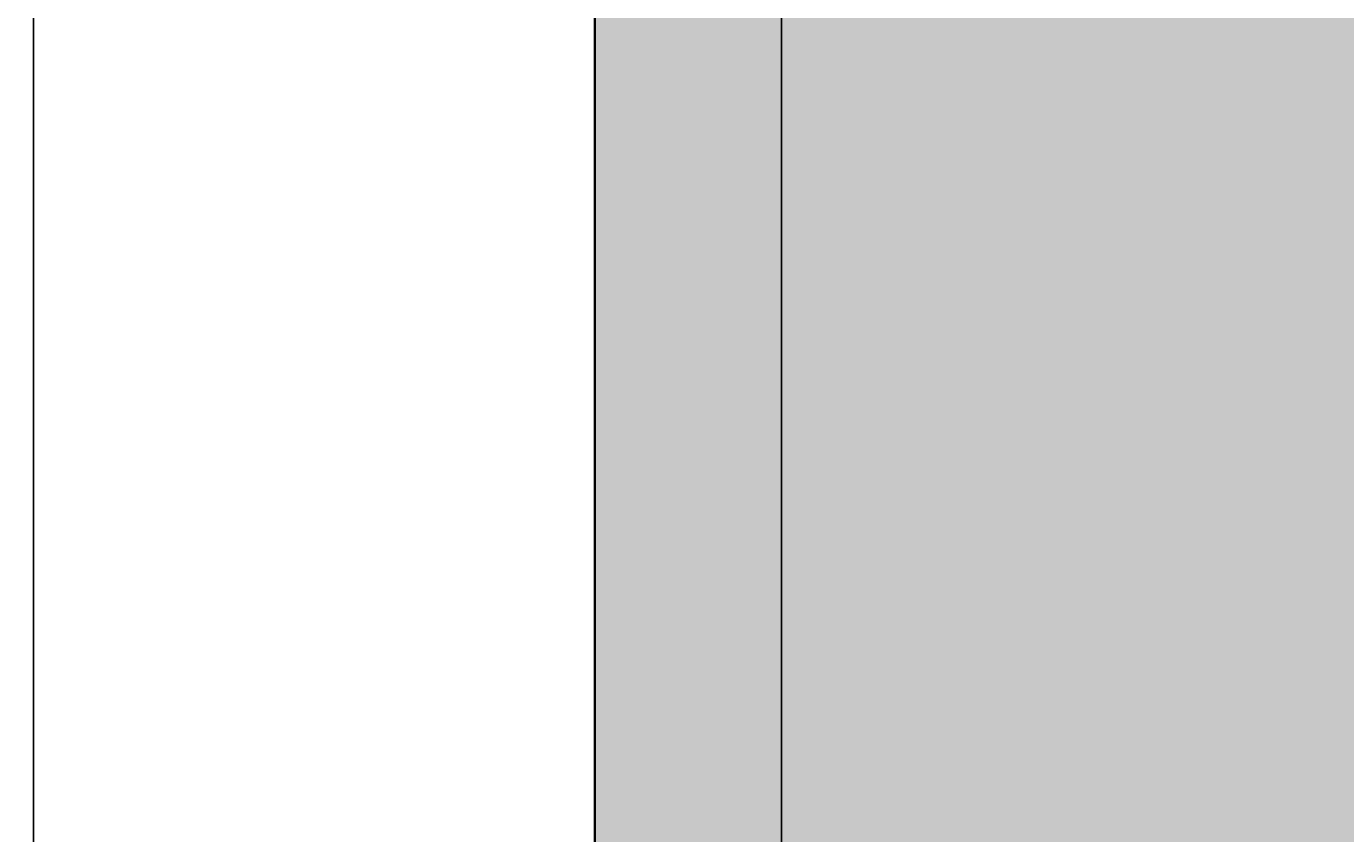
# Model space of a CAD drawing. Units: feet. Extents: x 2695 to 2912, y 795 to 1139.
# Tile 46 of 83: x 2695 to 2732, y 1071 to 1093. Entities that reach past the tile are written whole.
import ezdxf

# ---------------------------------------------------------------- set-up
doc = ezdxf.new("R2010")
doc.units = ezdxf.units.FT
for name, color, linetype, lineweight in [('A-ANNO-DIMS', 2, 'Continuous', 18), ('A-ELEV', 7, 'Continuous', 35), ('A-ELEV-PATT', 252, 'Continuous', 13)]:
    doc.layers.add(name, color=color, linetype=linetype, lineweight=lineweight)
doc.styles.get("Standard").update_dxf_attribs({"font": 'arial.ttf'})
doc.dimstyles.get("Standard").update_dxf_attribs({"dimtxt": 0.18, "dimasz": 0.18, "dimexe": 0.18, "dimexo": 0.0625, "dimgap": 0.09, "dimtad": 0, "dimtih": 1, "dimtoh": 1, "dimdec": 1, "dimzin": 0, "dimdsep": 46, "dimlunit": 3, "dimtxsty": 'Standard', "dimcen": 0.09, "dimadec": 0, "dimazin": 0, "dimtfac": 1, "dimtdec": 1, "dimtofl": 0, "dimtmove": 0, "dimatfit": 3, "dimfxl": 1, "dimtolj": 1, "dimtzin": 0, "dimarcsym": 0})

# ---------------------------------------------------------------- blocks, each defined once
blk = doc.blocks.new('*D7')
at = {"layer": 'A-ANNO-DIMS', "color": 0, "lineweight": -2, "transparency": 16777216}
for p, q in [((2710.636, 1122.993), (2710.636, 1138.886)), ((2715.885, 1050.373), (2715.885, 1138.886)), ((2710.816, 1138.706), (2712.867, 1138.706)), ((2715.705, 1138.706), (2713.655, 1138.706))]:
    blk.add_line(p, q, dxfattribs=at)
at = {"layer": 'A-ANNO-DIMS', "color": 0, "transparency": 16777216}
for points in [[(2710.816, 1138.736), (2710.816, 1138.676), (2710.636, 1138.706)], [(2715.705, 1138.736), (2715.705, 1138.676), (2715.885, 1138.706)]]:
    blk.add_solid(points, dxfattribs=at)
at = {"layer": 'Defpoints', "color": 0, "transparency": 16777216}
for p in [(2715.885, 1138.706), (2710.636, 1122.931), (2715.885, 1050.311)]:
    blk.add_point(p, dxfattribs=at)
at = {"layer": 'A-ANNO-DIMS', "color": 0, "transparency": 16777216, "insert": (2713.261, 1138.706), "char_height": 0.18, "attachment_point": 5}
blk.add_mtext('\\A1;5.249', dxfattribs=at)
blk = doc.blocks.new('*D8')
at = {"layer": 'A-ANNO-DIMS', "color": 0, "lineweight": -2, "transparency": 16777216}
for p, q in [((2715.885, 1050.373), (2715.885, 1138.886)), ((2770.636, 1122.993), (2770.636, 1138.886)), ((2716.065, 1138.706), (2742.866, 1138.706)), ((2770.456, 1138.706), (2743.655, 1138.706))]:
    blk.add_line(p, q, dxfattribs=at)
at = {"layer": 'A-ANNO-DIMS', "color": 0, "transparency": 16777216}
for points in [[(2716.065, 1138.736), (2716.065, 1138.676), (2715.885, 1138.706)], [(2770.456, 1138.736), (2770.456, 1138.676), (2770.636, 1138.706)]]:
    blk.add_solid(points, dxfattribs=at)
at = {"layer": 'Defpoints', "color": 0, "transparency": 16777216}
for p in [(2770.636, 1138.706), (2770.636, 1122.931), (2715.885, 1050.311)]:
    blk.add_point(p, dxfattribs=at)
at = {"layer": 'A-ANNO-DIMS', "color": 0, "transparency": 16777216, "insert": (2743.261, 1138.706), "char_height": 0.18, "attachment_point": 5}
blk.add_mtext('\\A1;54.75', dxfattribs=at)
blk = doc.blocks.new('*D12')
at = {"layer": 'A-ANNO-DIMS', "color": 0, "lineweight": -2, "transparency": 16777216}
for p, q in [((2710.574, 1122.931), (2694.681, 1122.931)), ((2694.861, 1122.751), (2694.861, 967.113)), ((2694.861, 811.111), (2694.861, 966.749)), ((2710.574, 810.931), (2694.681, 810.931))]:
    blk.add_line(p, q, dxfattribs=at)
at = {"layer": 'A-ANNO-DIMS', "color": 0, "transparency": 16777216}
for points in [[(2694.831, 1122.751), (2694.891, 1122.751), (2694.861, 1122.931)], [(2694.831, 811.111), (2694.891, 811.111), (2694.861, 810.931)]]:
    blk.add_solid(points, dxfattribs=at)
at = {"layer": 'Defpoints', "color": 0, "transparency": 16777216}
for p in [(2694.861, 1122.931), (2710.636, 1122.931), (2710.636, 810.931)]:
    blk.add_point(p, dxfattribs=at)
at = {"layer": 'A-ANNO-DIMS', "color": 0, "transparency": 16777216, "insert": (2694.861, 966.931), "char_height": 0.18, "attachment_point": 5}
blk.add_mtext('\\A1;312', dxfattribs=at)

msp = doc.modelspace()

# ---------------------------------------------------------------- hatches: boundary and pattern name
at = {"layer": 'A-ELEV-PATT'}
h = msp.add_hatch(color=256, dxfattribs=at)
h.set_gradient(color1=(147, 149, 152), color2=(147, 149, 152), tint=1)
h.paths.add_polyline_path([(2770.6361, 1118.4096), (2710.6361, 1118.4096), (2710.6361, 1062.9306), (2770.6361, 1062.9306)])
h.paths.add_polyline_path([(2890.6361, 1103.3378), (2770.6361, 1103.3378), (2770.6361, 1062.9306), (2890.6361, 1062.9306)])
h.paths.add_polyline_path([(2730.7081, 1048.1052), (2755.1125, 1048.1052), (2755.1125, 936.9306), (2770.6361, 936.9306), (2770.6361, 1050.3105), (2715.8852, 1050.3105), (2715.8852, 936.9306), (2730.7081, 936.9306)])
h.paths.add_polyline_path([(2890.6361, 1050.3105), (2770.6361, 1050.3105), (2770.6361, 971.9673), (2778.0341, 971.9673), (2778.0341, 1020.8235), (2843.575, 1020.8235), (2843.575, 971.9673), (2890.6361, 971.9673)])
h.paths.add_polyline_path([(2888.1882, 970.7156), (2843.575, 970.7156), (2843.575, 964.8267), (2888.1882, 964.8267)])
h.paths.add_polyline_path([(2888.1882, 964.1328), (2843.575, 964.1328), (2843.575, 956.614), (2888.1882, 956.614)])
h.paths.add_polyline_path([(2888.1882, 955.9202), (2843.575, 955.9202), (2843.575, 949.2892), (2888.1882, 949.2892)])
h.paths.add_polyline_path([(2888.1882, 948.5954), (2843.575, 948.5954), (2843.575, 941.3507), (2888.1882, 941.3507)])
h.paths.add_polyline_path([(2888.1882, 940.6569), (2843.575, 940.6569), (2843.575, 936.9306), (2888.1882, 936.9306)])
h.paths.add_polyline_path([(2890.6361, 970.7156), (2888.9368, 970.7156), (2888.9368, 964.8267), (2890.6361, 964.8267)])
h.paths.add_polyline_path([(2890.6361, 964.1328), (2888.9368, 964.1328), (2888.9368, 956.614), (2890.6361, 956.614)])
h.paths.add_polyline_path([(2890.6361, 955.9202), (2888.9368, 955.9202), (2888.9368, 949.2892), (2890.6361, 949.2892)])
h.paths.add_polyline_path([(2890.6361, 940.6569), (2888.9368, 940.6569), (2888.9368, 936.9306), (2890.6361, 936.9306)])
h.paths.add_polyline_path([(2890.6361, 948.5954), (2888.9368, 948.5954), (2888.9368, 941.3507), (2890.6361, 941.3507)])
h.paths.add_polyline_path([(2772.5216, 970.7156), (2770.6361, 970.7156), (2770.6361, 964.8267), (2772.5216, 964.8267)])
h.paths.add_polyline_path([(2772.5216, 964.1328), (2770.6361, 964.1328), (2770.6361, 956.614), (2772.5216, 956.614)])
h.paths.add_polyline_path([(2772.5216, 955.9202), (2770.6361, 955.9202), (2770.6361, 949.2892), (2772.5216, 949.2892)])
h.paths.add_polyline_path([(2772.5216, 948.5954), (2770.6361, 948.5954), (2770.6361, 941.3507), (2772.5216, 941.3507)])
h.paths.add_polyline_path([(2772.5216, 940.6569), (2770.6361, 940.6569), (2770.6361, 936.9306), (2772.5216, 936.9306)])
h.paths.add_polyline_path([(2778.0341, 940.6569), (2773.2702, 940.6569), (2773.2702, 936.9306), (2778.0341, 936.9306)])
h.paths.add_polyline_path([(2778.0341, 970.7156), (2773.2702, 970.7156), (2773.2702, 964.8267), (2778.0341, 964.8267)])
h.paths.add_polyline_path([(2778.0341, 964.1328), (2773.2702, 964.1328), (2773.2702, 956.614), (2778.0341, 956.614)])
h.paths.add_polyline_path([(2778.0341, 955.9202), (2773.2702, 955.9202), (2773.2702, 949.2892), (2778.0341, 949.2892)])
h.paths.add_polyline_path([(2778.0341, 948.5954), (2773.2702, 948.5954), (2773.2702, 941.3507), (2778.0341, 941.3507)])
h.paths.add_polyline_path([(2810.0407, 940.6569), (2780.0341, 940.6569), (2780.0341, 936.9306), (2810.0407, 936.9306)])
h.paths.add_polyline_path([(2890.6361, 924.3105), (2770.6361, 924.3105), (2770.6361, 810.9306), (2773.5029, 810.9306), (2773.5029, 905.5143), (2805.9398, 905.5143), (2838.3767, 905.5143), (2838.3767, 810.9306), (2890.6361, 810.9306)])

# ---------------------------------------------------------------- linework, layer by layer
at = {"layer": 'A-ELEV'}
for p, q in [((2710.6361, 1062.9306), (2710.6361, 1122.9306)), ((2710.6361, 1118.4096), (2710.6361, 1062.9306))]:
    msp.add_line(p, q, dxfattribs=at)

# ---------------------------------------------------------------- dimensions: what is measured, and where the dimension line sits
at = {"layer": 'A-ANNO-DIMS'}
for base, p1, p2, override, picture, middle in [((2715.8852, 1138.7056), (2710.6361, 1122.9306), (2715.8852, 1050.3105), {"dimdec": 3, "dimlfac": 1, "dimrnd": 0, "dimzin": 0, "dimdsep": 46, "dimlunit": 2}, '*D7', (2713.2606, 1138.7056)), ((2770.6361, 1138.7056), (2715.8852, 1050.3105), (2770.6361, 1122.9306), {"dimdec": 2, "dimlfac": 1, "dimrnd": 0, "dimzin": 0, "dimdsep": 46, "dimlunit": 2}, '*D8', (2743.2606, 1138.7056))]:
    dim = msp.add_linear_dim(base=base, p1=p1, p2=p2, dimstyle='Standard', override=override, dxfattribs=at)
    dim.commit()
    dim.dimension.update_dxf_attribs({"geometry": picture, "text_midpoint": middle})
dim = msp.add_linear_dim(base=(2694.8611, 1122.9306), p1=(2710.6361, 810.9306), p2=(2710.6361, 1122.9306), angle=90, dimstyle='Standard', override={"dimdec": 0, "dimlfac": 1, "dimrnd": 0, "dimzin": 0, "dimdsep": 46, "dimlunit": 2}, dxfattribs=at)
dim.commit()
dim.dimension.update_dxf_attribs({"geometry": '*D12', "text_midpoint": (2694.8611, 966.9306)})

doc.saveas('drawing.dxf')
